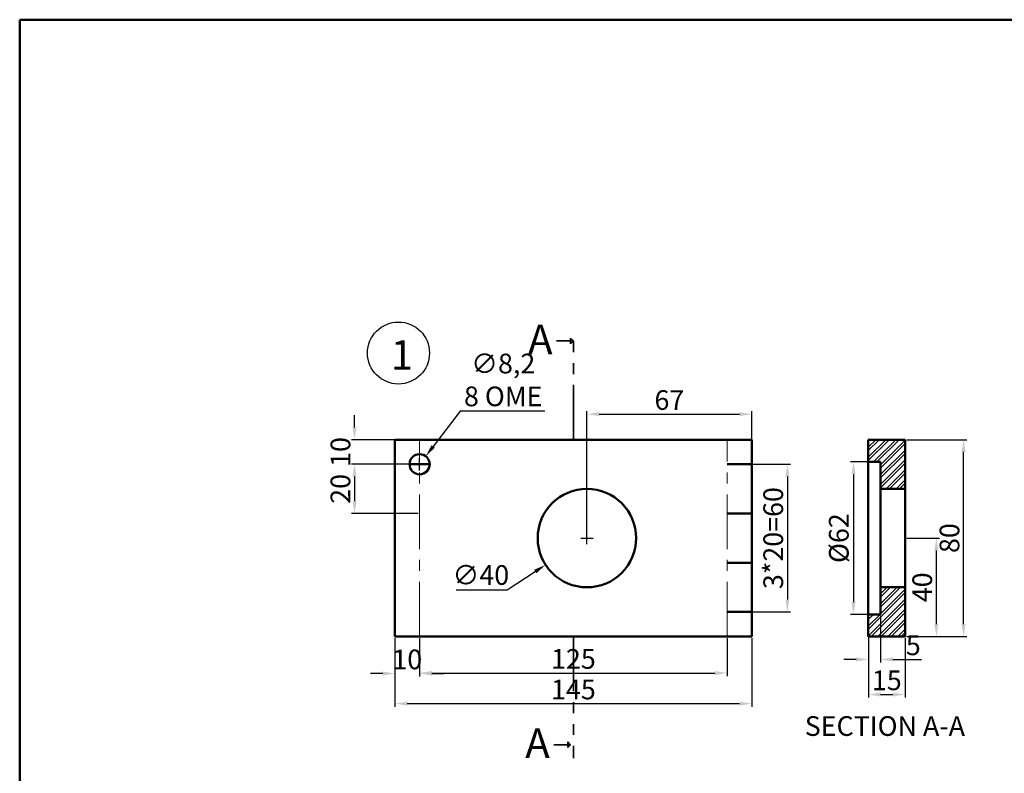
# Model space of a CAD drawing. Units: millimetres. Extents: x -749 to 333, y -22 to 680.
# Tile 2 of 4: x -749 to -349, y 374 to 680. Entities that reach past the tile are written whole.
import ezdxf

# ---------------------------------------------------------------- set-up
doc = ezdxf.new("R2010")
doc.units = ezdxf.units.MM
doc.header["$LTSCALE"] = 0.7
doc.linetypes.add('CENTER', pattern=[50.8, 31.75, -6.35, 6.35, -6.35])
doc.linetypes.add('PHANTOM', pattern=[63.5, 31.75, -6.35, 6.35, -6.35, 6.35, -6.35])
for name, color, linetype, lineweight in [('M-CNTR', 1, 'CENTER', 18), ('M-DIMS', 2, 'Continuous', 25), ('M-HATC', 8, 'Continuous', 18), ('M-OUTL', 7, 'Continuous', 50), ('M-SECT', 6, 'PHANTOM', 35), ('M-TEXT', 3, 'Continuous', 25), ('M-TTLB', 7, 'Continuous', 50)]:
    doc.layers.add(name, color=color, linetype=linetype, lineweight=lineweight)
doc.styles.get("Standard").update_dxf_attribs({"font": 'arial.ttf'})
doc.dimstyles.new('ISO-25', dxfattribs={"dimtxt": 8, "dimasz": 5, "dimexe": 1.25, "dimexo": 0.625, "dimtad": 1, "dimtoh": 1, "dimtxsty": 'Standard', "dimcen": 2.5, "dimadec": 0, "dimazin": 0, "dimtfac": 1, "dimtofl": 0, "dimtmove": 0, "dimatfit": 3, "dimfxl": 1, "dimarcsym": 0})

# ---------------------------------------------------------------- blocks, each defined once
blk = doc.blocks.new('*D1')
at = {"layer": 'Defpoints', "color": 0, "transparency": 16777216}
for p in [(-586.86, 509.24), (-613.29, 499.24), (-586.86, 499.24)]:
    blk.add_point(p, dxfattribs=at)
at = {"layer": 'M-DIMS', "color": 0, "lineweight": -2, "transparency": 16777216}
for p, q in [((-613.29, 514.24), (-613.29, 519.24)), ((-587.48, 509.24), (-614.54, 509.24)), ((-587.48, 499.24), (-614.54, 499.24)), ((-613.29, 494.24), (-613.29, 489.24))]:
    blk.add_line(p, q, dxfattribs=at)
at = {"layer": 'M-DIMS', "color": 0, "transparency": 16777216}
for points in [[(-614.12, 514.24), (-612.45, 514.24), (-613.29, 509.24)], [(-614.12, 494.24), (-612.45, 494.24), (-613.29, 499.24)]]:
    blk.add_solid(points, dxfattribs=at)
at = {"layer": 'M-DIMS', "color": 0, "transparency": 16777216, "insert": (-617.99, 504.24), "char_height": 8, "attachment_point": 5, "rotation": 90}
blk.add_mtext('10', dxfattribs=at)
blk = doc.blocks.new('*D2')
at = {"layer": 'Defpoints', "color": 0, "transparency": 16777216}
for p in [(-586.86, 499.24), (-613.29, 479.24), (-586.86, 479.24)]:
    blk.add_point(p, dxfattribs=at)
at = {"layer": 'M-DIMS', "color": 0, "lineweight": -2, "transparency": 16777216}
for p, q in [((-587.48, 499.24), (-614.54, 499.24)), ((-613.29, 494.24), (-613.29, 484.24)), ((-587.48, 479.24), (-614.54, 479.24))]:
    blk.add_line(p, q, dxfattribs=at)
at = {"layer": 'M-DIMS', "color": 0, "transparency": 16777216}
for points in [[(-614.12, 494.24), (-612.45, 494.24), (-613.29, 499.24)], [(-614.12, 484.24), (-612.45, 484.24), (-613.29, 479.24)]]:
    blk.add_solid(points, dxfattribs=at)
at = {"layer": 'M-DIMS', "color": 0, "transparency": 16777216, "insert": (-617.99, 489.24), "char_height": 8, "attachment_point": 5, "rotation": 90}
blk.add_mtext('20', dxfattribs=at)
blk = doc.blocks.new('*D3')
at = {"layer": 'Defpoints', "color": 0, "transparency": 16777216}
for p in [(-596.86, 429.24), (-586.86, 429.24), (-586.86, 414.21)]:
    blk.add_point(p, dxfattribs=at)
at = {"layer": 'M-DIMS', "color": 0, "lineweight": -2, "transparency": 16777216}
for p, q in [((-596.86, 428.62), (-596.86, 412.96)), ((-586.86, 428.62), (-586.86, 412.96)), ((-601.86, 414.21), (-606.86, 414.21)), ((-581.86, 414.21), (-576.86, 414.21))]:
    blk.add_line(p, q, dxfattribs=at)
at = {"layer": 'M-DIMS', "color": 0, "transparency": 16777216}
for points in [[(-601.86, 415.05), (-601.86, 413.38), (-596.86, 414.21)], [(-581.86, 415.05), (-581.86, 413.38), (-586.86, 414.21)]]:
    blk.add_solid(points, dxfattribs=at)
at = {"layer": 'M-DIMS', "color": 0, "transparency": 16777216, "insert": (-591.86, 418.92), "char_height": 8, "attachment_point": 5}
blk.add_mtext('10', dxfattribs=at)
blk = doc.blocks.new('*D4')
at = {"layer": 'Defpoints', "color": 0, "transparency": 16777216}
for p in [(-586.86, 429.24), (-461.86, 429.24), (-461.86, 414.41)]:
    blk.add_point(p, dxfattribs=at)
at = {"layer": 'M-DIMS', "color": 0, "lineweight": -2, "transparency": 16777216}
for p, q in [((-586.86, 428.62), (-586.86, 413.16)), ((-461.86, 428.62), (-461.86, 413.16)), ((-581.86, 414.41), (-466.86, 414.41))]:
    blk.add_line(p, q, dxfattribs=at)
at = {"layer": 'M-DIMS', "color": 0, "transparency": 16777216}
for points in [[(-581.86, 415.24), (-581.86, 413.57), (-586.86, 414.41)], [(-466.86, 415.24), (-466.86, 413.57), (-461.86, 414.41)]]:
    blk.add_solid(points, dxfattribs=at)
at = {"layer": 'M-DIMS', "color": 0, "transparency": 16777216, "insert": (-524.36, 419.12), "char_height": 8, "attachment_point": 5}
blk.add_mtext('125', dxfattribs=at)
blk = doc.blocks.new('*D5')
at = {"layer": 'Defpoints', "color": 0, "transparency": 16777216}
for p in [(-596.86, 429.24), (-451.86, 429.24), (-451.86, 401.98)]:
    blk.add_point(p, dxfattribs=at)
at = {"layer": 'M-DIMS', "color": 0, "lineweight": -2, "transparency": 16777216}
for p, q in [((-596.86, 428.62), (-596.86, 400.73)), ((-451.86, 428.62), (-451.86, 400.73)), ((-591.86, 401.98), (-456.86, 401.98))]:
    blk.add_line(p, q, dxfattribs=at)
at = {"layer": 'M-DIMS', "color": 0, "transparency": 16777216}
for points in [[(-591.86, 402.81), (-591.86, 401.14), (-596.86, 401.98)], [(-456.86, 402.81), (-456.86, 401.14), (-451.86, 401.98)]]:
    blk.add_solid(points, dxfattribs=at)
at = {"layer": 'M-DIMS', "color": 0, "transparency": 16777216, "insert": (-524.36, 406.68), "char_height": 8, "attachment_point": 5}
blk.add_mtext('145', dxfattribs=at)
blk = doc.blocks.new('*D6')
at = {"layer": 'Defpoints', "color": 0, "transparency": 16777216}
for p in [(-461.86, 499.24), (-461.86, 439.24), (-437.41, 439.24)]:
    blk.add_point(p, dxfattribs=at)
at = {"layer": 'M-DIMS', "color": 0, "lineweight": -2, "transparency": 16777216}
for p, q in [((-461.23, 499.24), (-436.16, 499.24)), ((-437.41, 494.24), (-437.41, 444.24)), ((-461.23, 439.24), (-436.16, 439.24))]:
    blk.add_line(p, q, dxfattribs=at)
at = {"layer": 'M-DIMS', "color": 0, "transparency": 16777216}
for points in [[(-438.24, 494.24), (-436.58, 494.24), (-437.41, 499.24)], [(-438.24, 444.24), (-436.58, 444.24), (-437.41, 439.24)]]:
    blk.add_solid(points, dxfattribs=at)
at = {"layer": 'M-DIMS', "color": 0, "transparency": 16777216, "insert": (-442.12, 469.24), "char_height": 8, "attachment_point": 5, "rotation": 90}
blk.add_mtext('3*20=60', dxfattribs=at)
blk = doc.blocks.new('*D7')
at = {"layer": 'Defpoints', "color": 0, "transparency": 16777216}
for p in [(-502.06, 480.1), (-535.65, 458.38)]:
    blk.add_point(p, dxfattribs=at)
at = {"layer": 'M-DIMS', "color": 0, "lineweight": -2, "transparency": 16777216}
for p, q in [((-521.36, 469.24), (-516.36, 469.24)), ((-518.86, 466.74), (-518.86, 471.74)), ((-551.29, 448.27), (-539.85, 455.67)), ((-572.05, 448.27), (-551.29, 448.27))]:
    blk.add_line(p, q, dxfattribs=at)
at = {"layer": 'M-DIMS', "color": 0, "transparency": 16777216}
blk.add_solid([(-540.3, 456.37), (-539.4, 454.97), (-535.65, 458.38)], dxfattribs=at)
at = {"layer": 'M-DIMS', "color": 0, "transparency": 16777216, "insert": (-561.98, 453.21), "char_height": 8, "attachment_point": 5}
blk.add_mtext('∅40', dxfattribs=at)
blk = doc.blocks.new('*D8')
at = {"layer": 'Defpoints', "color": 0, "transparency": 16777216}
for p in [(-584.37, 502.5), (-589.34, 495.98)]:
    blk.add_point(p, dxfattribs=at)
at = {"layer": 'M-DIMS', "color": 0, "lineweight": -2, "transparency": 16777216}
for p, q in [((-570.37, 520.89), (-581.34, 506.48)), ((-536.02, 520.89), (-570.37, 520.89)), ((-586.86, 496.74), (-586.86, 501.74)), ((-589.36, 499.24), (-584.36, 499.24))]:
    blk.add_line(p, q, dxfattribs=at)
at = {"layer": 'M-DIMS', "color": 0, "transparency": 16777216}
blk.add_solid([(-582.01, 506.99), (-580.68, 505.98), (-584.37, 502.5)], dxfattribs=at)
at = {"layer": 'M-DIMS', "color": 0, "transparency": 16777216, "insert": (-552.88, 532.47), "char_height": 8, "attachment_point": 5}
blk.add_mtext('∅8,2\\P8 OME', dxfattribs=at)
blk = doc.blocks.new('*D9')
at = {"layer": 'Defpoints', "color": 0, "transparency": 16777216}
for p in [(-402.01, 500.24), (-410.54, 438.24), (-402.01, 438.24)]:
    blk.add_point(p, dxfattribs=at)
at = {"layer": 'M-DIMS', "color": 0, "lineweight": -2, "transparency": 16777216}
for p, q in [((-402.64, 500.24), (-411.79, 500.24)), ((-410.54, 495.24), (-410.54, 443.24)), ((-402.64, 438.24), (-411.79, 438.24))]:
    blk.add_line(p, q, dxfattribs=at)
at = {"layer": 'M-DIMS', "color": 0, "transparency": 16777216}
for points in [[(-411.37, 495.24), (-409.7, 495.24), (-410.54, 500.24)], [(-411.37, 443.24), (-409.7, 443.24), (-410.54, 438.24)]]:
    blk.add_solid(points, dxfattribs=at)
at = {"layer": 'M-DIMS', "color": 0, "transparency": 16777216, "insert": (-415.47, 469.24), "char_height": 8, "attachment_point": 5, "rotation": 90}
blk.add_mtext('%%C62', dxfattribs=at)
blk = doc.blocks.new('*D10')
at = {"layer": 'Defpoints', "color": 0, "transparency": 16777216}
for p in [(-389.51, 469.24), (-376.86, 469.24), (-389.51, 429.24)]:
    blk.add_point(p, dxfattribs=at)
at = {"layer": 'M-DIMS', "color": 0, "lineweight": -2, "transparency": 16777216}
for p, q in [((-388.89, 469.24), (-375.61, 469.24)), ((-376.86, 434.24), (-376.86, 464.24)), ((-388.89, 429.24), (-375.61, 429.24))]:
    blk.add_line(p, q, dxfattribs=at)
at = {"layer": 'M-DIMS', "color": 0, "transparency": 16777216}
for points in [[(-377.7, 464.24), (-376.03, 464.24), (-376.86, 469.24)], [(-377.7, 434.24), (-376.03, 434.24), (-376.86, 429.24)]]:
    blk.add_solid(points, dxfattribs=at)
at = {"layer": 'M-DIMS', "color": 0, "transparency": 16777216, "insert": (-381.57, 449.24), "char_height": 8, "attachment_point": 5, "rotation": 90}
blk.add_mtext('40', dxfattribs=at)
blk = doc.blocks.new('*D11')
at = {"layer": 'Defpoints', "color": 0, "transparency": 16777216}
for p in [(-389.51, 509.24), (-365.79, 509.24), (-389.51, 429.24)]:
    blk.add_point(p, dxfattribs=at)
at = {"layer": 'M-DIMS', "color": 0, "lineweight": -2, "transparency": 16777216}
for p, q in [((-388.89, 509.24), (-364.54, 509.24)), ((-365.79, 434.24), (-365.79, 504.24)), ((-388.89, 429.24), (-364.54, 429.24))]:
    blk.add_line(p, q, dxfattribs=at)
at = {"layer": 'M-DIMS', "color": 0, "transparency": 16777216}
for points in [[(-366.63, 504.24), (-364.96, 504.24), (-365.79, 509.24)], [(-366.63, 434.24), (-364.96, 434.24), (-365.79, 429.24)]]:
    blk.add_solid(points, dxfattribs=at)
at = {"layer": 'M-DIMS', "color": 0, "transparency": 16777216, "insert": (-370.5, 469.24), "char_height": 8, "attachment_point": 5, "rotation": 90}
blk.add_mtext('80', dxfattribs=at)
blk = doc.blocks.new('*D12')
at = {"layer": 'Defpoints', "color": 0, "transparency": 16777216}
for p in [(-404.51, 429.24), (-389.51, 429.24), (-389.51, 405.7)]:
    blk.add_point(p, dxfattribs=at)
at = {"layer": 'M-DIMS', "color": 0, "lineweight": -2, "transparency": 16777216}
for p, q in [((-404.51, 428.62), (-404.51, 404.45)), ((-389.51, 428.62), (-389.51, 404.45)), ((-399.51, 405.7), (-394.51, 405.7))]:
    blk.add_line(p, q, dxfattribs=at)
at = {"layer": 'M-DIMS', "color": 0, "transparency": 16777216}
for points in [[(-399.51, 406.53), (-399.51, 404.86), (-404.51, 405.7)], [(-394.51, 406.53), (-394.51, 404.86), (-389.51, 405.7)]]:
    blk.add_solid(points, dxfattribs=at)
at = {"layer": 'M-DIMS', "color": 0, "transparency": 16777216, "insert": (-397.01, 410.41), "char_height": 8, "attachment_point": 5}
blk.add_mtext('15', dxfattribs=at)
blk = doc.blocks.new('*D13')
at = {"layer": 'Defpoints', "color": 0, "transparency": 16777216}
for p in [(-404.51, 438.24), (-399.51, 438.24), (-399.51, 419.94)]:
    blk.add_point(p, dxfattribs=at)
at = {"layer": 'M-DIMS', "color": 0, "lineweight": -2, "transparency": 16777216}
for p, q in [((-404.51, 437.62), (-404.51, 418.69)), ((-399.51, 437.62), (-399.51, 418.69)), ((-409.51, 419.94), (-414.51, 419.94)), ((-394.51, 419.94), (-382.96, 419.94))]:
    blk.add_line(p, q, dxfattribs=at)
at = {"layer": 'M-DIMS', "color": 0, "transparency": 16777216}
for points in [[(-409.51, 420.77), (-409.51, 419.11), (-404.51, 419.94)], [(-394.51, 420.77), (-394.51, 419.11), (-399.51, 419.94)]]:
    blk.add_solid(points, dxfattribs=at)
at = {"layer": 'M-DIMS', "color": 0, "transparency": 16777216, "insert": (-386.24, 424.63), "char_height": 8, "attachment_point": 5}
blk.add_mtext('5', dxfattribs=at)
blk = doc.blocks.new('*D87')
at = {"layer": 'Defpoints', "color": 0, "transparency": 16777216}
for p in [(-451.86, 519.61), (-518.86, 469.24), (-451.86, 469.24)]:
    blk.add_point(p, dxfattribs=at)
at = {"layer": 'M-DIMS', "color": 0, "lineweight": -2, "transparency": 16777216}
for p, q in [((-518.86, 469.87), (-518.86, 520.86)), ((-451.86, 469.87), (-451.86, 520.86)), ((-513.86, 519.61), (-456.86, 519.61))]:
    blk.add_line(p, q, dxfattribs=at)
at = {"layer": 'M-DIMS', "color": 0, "transparency": 16777216}
for points in [[(-513.86, 520.44), (-513.86, 518.78), (-518.86, 519.61)], [(-456.86, 520.44), (-456.86, 518.78), (-451.86, 519.61)]]:
    blk.add_solid(points, dxfattribs=at)
at = {"layer": 'M-DIMS', "color": 0, "transparency": 16777216, "insert": (-485.36, 524.32), "char_height": 8, "attachment_point": 5}
blk.add_mtext('67', dxfattribs=at)
blk = doc.blocks.new('HOLE-8')
blk.add_line((0, 4.1), (8.2, 4.1))
blk.add_circle((4.1, 4.1), 4.1)

msp = doc.modelspace()

# ---------------------------------------------------------------- hatches: boundary and pattern name
at = {"layer": 'M-HATC'}
h = msp.add_hatch(dxfattribs=at)
h.set_pattern_fill('ANSI32', color=256, scale=0.3)
h.set_pattern_definition([(45, (-3233.924, -565.3363), (-2.0205576, 2.0205576), []), (45, (-3232.5768, -565.3363), (-2.0205576, 2.0205576), [])])
h.paths.add_polyline_path([(-399.514, 509.242), (-404.514, 509.242), (-404.514, 500.242), (-399.514, 500.242), (-399.514, 489.242), (-389.514, 489.242), (-389.514, 509.242)])
h.paths.add_polyline_path([(-389.514, 449.242), (-399.514, 449.242), (-399.514, 438.242), (-404.514, 438.242), (-404.514, 429.242), (-399.514, 429.242), (-389.514, 429.242)])

# ---------------------------------------------------------------- linework, layer by layer
at = {"layer": 'M-CNTR'}
for p, q in [((-586.857, 429.242), (-586.857, 509.242)), ((-461.857, 429.242), (-461.857, 509.242))]:
    msp.add_line(p, q, dxfattribs=at)
at = {"layer": 'M-OUTL'}
for p, q in [((-596.857, 509.242), (-451.857, 509.242)), ((-596.857, 429.242), (-596.857, 509.242)), ((-451.857, 429.242), (-451.857, 509.242)), ((-404.514, 509.242), (-399.514, 509.242)), ((-404.514, 500.242), (-404.514, 509.242)), ((-399.514, 509.242), (-389.514, 509.242)), ((-389.514, 509.242), (-389.514, 469.242)), ((-399.514, 500.242), (-404.514, 500.242)), ((-404.514, 438.242), (-404.514, 500.242)), ((-399.514, 469.242), (-399.514, 500.242)), ((-461.857, 499.242), (-451.857, 499.242)), ((-399.514, 479.242), (-399.514, 499.242)), ((-389.514, 489.242), (-399.514, 489.242)), ((-461.857, 479.242), (-451.857, 479.242)), ((-399.514, 469.242), (-399.514, 438.242)), ((-389.514, 429.242), (-389.514, 469.242)), ((-461.857, 459.242), (-451.857, 459.242)), ((-399.514, 459.242), (-399.514, 439.242)), ((-389.514, 449.242), (-399.514, 449.242)), ((-461.857, 439.242), (-451.857, 439.242)), ((-399.514, 438.242), (-404.514, 438.242)), ((-404.514, 438.242), (-404.514, 429.242)), ((-596.857, 429.242), (-451.857, 429.242)), ((-404.514, 429.242), (-399.514, 429.242)), ((-399.514, 429.242), (-389.514, 429.242))]:
    msp.add_line(p, q, dxfattribs=at)
msp.add_circle((-518.857, 469.242), 20, dxfattribs=at)
at = {"layer": 'M-SECT'}
for p, q in [((-524.357, 509.242), (-524.357, 553.088)), ((-531.227, 549.385), (-524.357, 549.385)), ((-524.357, 549.385), (-525.494, 550.522)), ((-525.494, 550.522), (-525.494, 549.385)), ((-524.357, 549.385), (-525.494, 548.249)), ((-525.494, 548.249), (-525.494, 549.385)), ((-524.357, 429.242), (-524.357, 379.885)), ((-532.364, 385.286), (-525.494, 385.286)), ((-525.494, 385.286), (-526.63, 386.422)), ((-526.63, 386.422), (-526.63, 385.286)), ((-525.494, 385.286), (-526.63, 384.15)), ((-526.63, 384.15), (-526.63, 385.286))]:
    msp.add_line(p, q, dxfattribs=at)
at = {"layer": 'M-TEXT'}
msp.add_circle((-595.44, 544.453), 12.598, dxfattribs=at)
at = {"layer": 'M-TTLB', "ltscale": 0.7}
msp.add_lwpolyline([(-749.362, 679.91), (332.782, 679.91), (332.782, -22.287), (-749.362, -22.287)], close=True, dxfattribs=at)

# ---------------------------------------------------------------- block references
at = {"layer": 'M-OUTL'}
msp.add_blockref('HOLE-8', (-590.957, 495.142), dxfattribs=at)

# ---------------------------------------------------------------- texts
at = {"layer": 'M-TEXT', "attachment_point": 1}
for s, width, insert, char_height in [('A', 30.10277, (-542.795, 555.984), 12), ('1', 30.10277, (-598.588, 549.672), 12), ('SECTION A-A', 95.89335, (-430.365, 396.875), 8), ('A', 30.10277, (-543.931, 391.885), 12)]:
    msp.add_mtext_dynamic_manual_height_columns(s, width=width, gutter_width=12.5, heights=[0], dxfattribs=dict(at, insert=insert, char_height=char_height))

# ---------------------------------------------------------------- dimensions: what is measured, and where the dimension line sits
at = {"layer": 'M-DIMS'}
dim = msp.add_diameter_dim_2p(p1=(-589.342, 495.981), p2=(-584.373, 502.504), text='<>\\P8 OME', dimstyle='ISO-25', override={"dimclrd": 0, "dimclre": 0, "dimclrt": 0}, dxfattribs=at)
dim.commit()
dim.dimension.update_dxf_attribs({"geometry": '*D8', "text_midpoint": (-552.879, 520.888), "dimtype": 163})
for base, p1, p2, picture, middle in [((-451.857, 519.609), (-518.857, 469.242), (-451.857, 469.242), '*D87', (-485.357, 524.318)), ((-399.514, 419.939), (-404.514, 438.242), (-399.514, 438.242), '*D13', (-386.237, 424.632)), ((-451.857, 401.975), (-596.857, 429.242), (-451.857, 429.242), '*D5', (-524.357, 406.685))]:
    dim = msp.add_linear_dim(base=base, p1=p1, p2=p2, dimstyle='ISO-25', override={"dimclrd": 0, "dimclre": 0, "dimclrt": 0}, dxfattribs=at)
    dim.commit()
    dim.dimension.update_dxf_attribs({"geometry": picture, "text_midpoint": middle})
for base, p1, p2, picture, middle in [((-613.285, 499.242), (-586.857, 509.242), (-586.857, 499.242), '*D1', (-613.285, 504.242)), ((-376.863, 469.242), (-389.514, 429.242), (-389.514, 469.242), '*D10', (-376.863, 449.242))]:
    dim = msp.add_linear_dim(base=base, p1=p1, p2=p2, angle=90, dimstyle='ISO-25', override={"dimclrd": 0, "dimclre": 0, "dimclrt": 0}, dxfattribs=at)
    dim.commit()
    dim.dimension.update_dxf_attribs({"geometry": picture, "text_midpoint": middle, "dimtype": 160})
for base, p1, p2, picture, middle in [((-365.792, 509.242), (-389.514, 429.242), (-389.514, 509.242), '*D11', (-370.501, 469.242)), ((-613.285, 479.242), (-586.857, 499.242), (-586.857, 479.242), '*D2', (-617.995, 489.242))]:
    dim = msp.add_linear_dim(base=base, p1=p1, p2=p2, angle=90, dimstyle='ISO-25', override={"dimclrd": 0, "dimclre": 0, "dimclrt": 0}, dxfattribs=at)
    dim.commit()
    dim.dimension.update_dxf_attribs({"geometry": picture, "text_midpoint": middle})
for base, p1, p2, text, picture, middle in [((-410.538, 438.242), (-402.014, 500.242), (-402.014, 438.242), '%%C<>', '*D9', (-415.471, 469.242)), ((-437.41, 439.242), (-461.857, 499.242), (-461.857, 439.242), '3*20=<>', '*D6', (-442.122, 469.242))]:
    dim = msp.add_linear_dim(base=base, p1=p1, p2=p2, angle=90, text=text, dimstyle='ISO-25', override={"dimclrd": 0, "dimclre": 0, "dimclrt": 0}, dxfattribs=at)
    dim.commit()
    dim.dimension.update_dxf_attribs({"geometry": picture, "text_midpoint": middle})
dim = msp.add_diameter_dim_2p(p1=(-502.062, 480.102), p2=(-535.652, 458.383), dimstyle='ISO-25', override={"dimclrd": 0, "dimclre": 0, "dimclrt": 0}, dxfattribs=at)
dim.commit()
dim.dimension.update_dxf_attribs({"geometry": '*D7', "text_midpoint": (-561.979, 453.208)})
for base, p1, p2, picture, middle in [((-586.857, 414.214), (-596.857, 429.242), (-586.857, 429.242), '*D3', (-591.857, 414.214)), ((-461.857, 414.408), (-586.857, 429.242), (-461.857, 429.242), '*D4', (-524.357, 414.408)), ((-389.514, 405.697), (-404.514, 429.242), (-389.514, 429.242), '*D12', (-397.014, 405.697))]:
    dim = msp.add_linear_dim(base=base, p1=p1, p2=p2, dimstyle='ISO-25', override={"dimclrd": 0, "dimclre": 0, "dimclrt": 0}, dxfattribs=at)
    dim.commit()
    dim.dimension.update_dxf_attribs({"geometry": picture, "text_midpoint": middle, "dimtype": 160})

doc.saveas('drawing.dxf')
